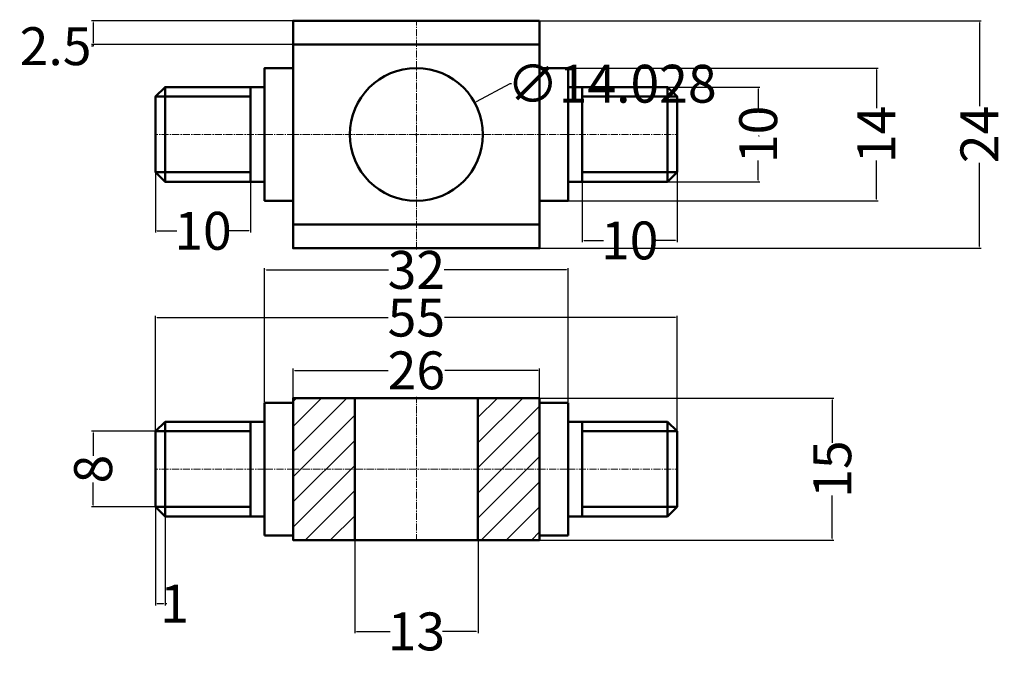
# Model space of a CAD drawing. Units: millimetres. Extents: x 37 to 141, y 13 to 80.
import ezdxf

# ---------------------------------------------------------------- set-up
doc = ezdxf.new("R2010")
doc.units = ezdxf.units.MM
doc.header["$MEASUREMENT"] = 0
doc.linetypes.add('CENTER2', pattern=[1.125, 0.75, -0.125, 0.125, -0.125])
for name, color, linetype, lineweight in [('M-CNTR', 4, 'CENTER2', 18), ('M-DIMS', 2, 'Continuous', 25), ('M-HATC', 8, 'Continuous', 18), ('M-OUTL', 7, 'Continuous', 50), ('M-TEXT', 7, 'Continuous', 25)]:
    doc.layers.add(name, color=color, linetype=linetype, lineweight=lineweight)
doc.styles.get("Standard").update_dxf_attribs({"font": 'arial.ttf'})
doc.dimstyles.get("Standard").update_dxf_attribs({"dimtxt": 4, "dimasz": 0.18, "dimexe": 0.18, "dimexo": 0.0625, "dimgap": 0.09, "dimtad": 0, "dimtoh": 1, "dimdec": 0, "dimzin": 0, "dimdsep": 46, "dimtxsty": 'Standard', "dimcen": 0.09, "dimadec": 0, "dimazin": 0, "dimtfac": 1, "dimtdec": 0, "dimtofl": 0, "dimtmove": 0, "dimatfit": 3, "dimfxl": 1, "dimtolj": 1, "dimtzin": 0, "dimarcsym": 0})

# ---------------------------------------------------------------- blocks, each defined once
blk = doc.blocks.new('*U1')
at = {"layer": 'M-CNTR', "color": 0, "transparency": 16777216}
blk.add_line((-1.62, 0), (1.62, 0), dxfattribs=at)
blk = doc.blocks.new('*U2')
at = {"layer": 'M-CNTR', "color": 0, "transparency": 16777216}
blk.add_line((0, -12.12), (0, 12.12), dxfattribs=at)
blk = doc.blocks.new('*U3')
at = {"layer": 'M-CNTR', "color": 0, "transparency": 16777216}
blk.add_line((-13.12, 0), (13.12, 0), dxfattribs=at)
blk = doc.blocks.new('*U4')
at = {"layer": 'M-CNTR', "color": 0, "transparency": 16777216}
blk.add_line((1.62, 0), (-1.62, 0), dxfattribs=at)
blk = doc.blocks.new('*U5')
at = {"layer": 'M-CNTR', "color": 0, "transparency": 16777216}
blk.add_line((1.62, 0), (-1.62, 0), dxfattribs=at)
blk = doc.blocks.new('*U6')
at = {"layer": 'M-CNTR', "color": 0, "transparency": 16777216}
blk.add_line((-1.62, 0), (1.62, 0), dxfattribs=at)
blk = doc.blocks.new('*U7')
at = {"layer": 'M-CNTR', "color": 0, "transparency": 16777216}
blk.add_line((-13.12, 0), (13.12, 0), dxfattribs=at)
blk = doc.blocks.new('*D8')
at = {"layer": 'Defpoints', "color": 0, "transparency": 16777216}
for p in [(78.94, 39.78), (78.94, 24.78), (122.8, 24.78)]:
    blk.add_point(p, dxfattribs=at)
at = {"layer": 'M-DIMS', "color": 0, "lineweight": -2, "transparency": 16777216}
for p, q in [((79, 39.78), (122.98, 39.78)), ((122.8, 39.6), (122.8, 35.06)), ((122.8, 24.96), (122.8, 29.5)), ((79, 24.78), (122.98, 24.78))]:
    blk.add_line(p, q, dxfattribs=at)
at = {"layer": 'M-DIMS', "color": 0, "transparency": 16777216}
for points in [[(122.77, 39.6), (122.83, 39.6), (122.8, 39.78)], [(122.77, 24.96), (122.83, 24.96), (122.8, 24.78)]]:
    blk.add_solid(points, dxfattribs=at)
at = {"layer": 'M-DIMS', "color": 0, "transparency": 16777216, "insert": (122.8, 32.28), "char_height": 4, "attachment_point": 5, "rotation": 90}
blk.add_mtext('\\A1;15', dxfattribs=at)
blk = doc.blocks.new('*D9')
at = {"layer": 'Defpoints', "color": 0, "transparency": 16777216}
for p in [(106.44, 48.27), (51.44, 32.28), (106.44, 32.28)]:
    blk.add_point(p, dxfattribs=at)
at = {"layer": 'M-DIMS', "color": 0, "lineweight": -2, "transparency": 16777216}
for p, q in [((51.44, 32.34), (51.44, 48.45)), ((51.62, 48.27), (75.97, 48.27)), ((106.26, 48.27), (81.91, 48.27)), ((106.44, 32.34), (106.44, 48.45))]:
    blk.add_line(p, q, dxfattribs=at)
at = {"layer": 'M-DIMS', "color": 0, "transparency": 16777216}
for points in [[(51.62, 48.3), (51.62, 48.24), (51.44, 48.27)], [(106.26, 48.3), (106.26, 48.24), (106.44, 48.27)]]:
    blk.add_solid(points, dxfattribs=at)
at = {"layer": 'M-DIMS', "color": 0, "transparency": 16777216, "insert": (78.94, 48.27), "char_height": 4, "attachment_point": 5}
blk.add_mtext('\\A1;55', dxfattribs=at)
blk = doc.blocks.new('*D10')
at = {"layer": 'Defpoints', "color": 0, "transparency": 16777216}
for p in [(94.94, 53.3), (62.94, 39.28), (94.94, 39.28)]:
    blk.add_point(p, dxfattribs=at)
at = {"layer": 'M-DIMS', "color": 0, "lineweight": -2, "transparency": 16777216}
for p, q in [((62.94, 39.34), (62.94, 53.48)), ((63.12, 53.3), (76.01, 53.3)), ((94.76, 53.3), (81.87, 53.3)), ((94.94, 39.34), (94.94, 53.48))]:
    blk.add_line(p, q, dxfattribs=at)
at = {"layer": 'M-DIMS', "color": 0, "transparency": 16777216}
for points in [[(63.12, 53.33), (63.12, 53.27), (62.94, 53.3)], [(94.76, 53.33), (94.76, 53.27), (94.94, 53.3)]]:
    blk.add_solid(points, dxfattribs=at)
at = {"layer": 'M-DIMS', "color": 0, "transparency": 16777216, "insert": (78.94, 53.3), "char_height": 4, "attachment_point": 5}
blk.add_mtext('\\A1;32', dxfattribs=at)
blk = doc.blocks.new('*D11')
at = {"layer": 'Defpoints', "color": 0, "transparency": 16777216}
for p in [(91.94, 42.7), (65.94, 39.78), (91.94, 39.78)]:
    blk.add_point(p, dxfattribs=at)
at = {"layer": 'M-DIMS', "color": 0, "lineweight": -2, "transparency": 16777216}
for p, q in [((65.94, 39.84), (65.94, 42.88)), ((66.12, 42.7), (75.95, 42.7)), ((91.76, 42.7), (81.93, 42.7)), ((91.94, 39.84), (91.94, 42.88))]:
    blk.add_line(p, q, dxfattribs=at)
at = {"layer": 'M-DIMS', "color": 0, "transparency": 16777216}
for points in [[(66.12, 42.73), (66.12, 42.67), (65.94, 42.7)], [(91.76, 42.73), (91.76, 42.67), (91.94, 42.7)]]:
    blk.add_solid(points, dxfattribs=at)
at = {"layer": 'M-DIMS', "color": 0, "transparency": 16777216, "insert": (78.94, 42.7), "char_height": 4, "attachment_point": 5}
blk.add_mtext('\\A1;26', dxfattribs=at)
blk = doc.blocks.new('*D12')
at = {"layer": 'Defpoints', "color": 0, "transparency": 16777216}
for p in [(72.44, 24.78), (85.44, 24.78), (85.44, 15.15)]:
    blk.add_point(p, dxfattribs=at)
at = {"layer": 'M-DIMS', "color": 0, "lineweight": -2, "transparency": 16777216}
for p, q in [((72.44, 24.72), (72.44, 14.97)), ((85.44, 24.72), (85.44, 14.97)), ((72.62, 15.15), (76.17, 15.15)), ((85.26, 15.15), (81.7, 15.15))]:
    blk.add_line(p, q, dxfattribs=at)
at = {"layer": 'M-DIMS', "color": 0, "transparency": 16777216}
for points in [[(72.62, 15.18), (72.62, 15.12), (72.44, 15.15)], [(85.26, 15.18), (85.26, 15.12), (85.44, 15.15)]]:
    blk.add_solid(points, dxfattribs=at)
at = {"layer": 'M-DIMS', "color": 0, "transparency": 16777216, "insert": (78.94, 15.15), "char_height": 4, "attachment_point": 5}
blk.add_mtext('\\A1;13', dxfattribs=at)
blk = doc.blocks.new('*D13')
at = {"layer": 'Defpoints', "color": 0, "transparency": 16777216}
for p in [(51.44, 63.6), (61.44, 63.6), (61.44, 57.43)]:
    blk.add_point(p, dxfattribs=at)
at = {"layer": 'M-DIMS', "color": 0, "lineweight": -2, "transparency": 16777216}
for p, q in [((51.44, 63.54), (51.44, 57.25)), ((61.44, 63.54), (61.44, 57.25)), ((51.62, 57.43), (53.68, 57.43)), ((61.26, 57.43), (59.2, 57.43))]:
    blk.add_line(p, q, dxfattribs=at)
at = {"layer": 'M-DIMS', "color": 0, "transparency": 16777216}
for points in [[(51.62, 57.46), (51.62, 57.4), (51.44, 57.43)], [(61.26, 57.46), (61.26, 57.4), (61.44, 57.43)]]:
    blk.add_solid(points, dxfattribs=at)
at = {"layer": 'M-DIMS', "color": 0, "transparency": 16777216, "insert": (56.44, 57.43), "char_height": 4, "attachment_point": 5}
blk.add_mtext('\\A1;10', dxfattribs=at)
blk = doc.blocks.new('*D14')
at = {"layer": 'Defpoints', "color": 0, "transparency": 16777216}
for p in [(96.44, 63.6), (106.44, 63.6), (106.44, 56.41)]:
    blk.add_point(p, dxfattribs=at)
at = {"layer": 'M-DIMS', "color": 0, "lineweight": -2, "transparency": 16777216}
for p, q in [((96.44, 63.54), (96.44, 56.23)), ((106.44, 63.54), (106.44, 56.23)), ((96.62, 56.41), (98.68, 56.41)), ((106.26, 56.41), (104.2, 56.41))]:
    blk.add_line(p, q, dxfattribs=at)
at = {"layer": 'M-DIMS', "color": 0, "transparency": 16777216}
for points in [[(96.62, 56.44), (96.62, 56.38), (96.44, 56.41)], [(106.26, 56.44), (106.26, 56.38), (106.44, 56.41)]]:
    blk.add_solid(points, dxfattribs=at)
at = {"layer": 'M-DIMS', "color": 0, "transparency": 16777216, "insert": (101.44, 56.41), "char_height": 4, "attachment_point": 5}
blk.add_mtext('\\A1;10', dxfattribs=at)
blk = doc.blocks.new('*D15')
at = {"layer": 'Defpoints', "color": 0, "transparency": 16777216}
for p in [(94.94, 74.6), (94.94, 60.6), (127.45, 60.6)]:
    blk.add_point(p, dxfattribs=at)
at = {"layer": 'M-DIMS', "color": 0, "lineweight": -2, "transparency": 16777216}
for p, q in [((95, 74.6), (127.63, 74.6)), ((127.45, 74.42), (127.45, 70.36)), ((127.45, 60.78), (127.45, 64.84)), ((95, 60.6), (127.63, 60.6))]:
    blk.add_line(p, q, dxfattribs=at)
at = {"layer": 'M-DIMS', "color": 0, "transparency": 16777216}
for points in [[(127.42, 74.42), (127.48, 74.42), (127.45, 74.6)], [(127.42, 60.78), (127.48, 60.78), (127.45, 60.6)]]:
    blk.add_solid(points, dxfattribs=at)
at = {"layer": 'M-DIMS', "color": 0, "transparency": 16777216, "insert": (127.45, 67.6), "char_height": 4, "attachment_point": 5, "rotation": 90}
blk.add_mtext('\\A1;14', dxfattribs=at)
blk = doc.blocks.new('*D16')
at = {"layer": 'Defpoints', "color": 0, "transparency": 16777216}
for p in [(91.94, 79.59), (91.94, 55.59), (138.32, 55.59)]:
    blk.add_point(p, dxfattribs=at)
at = {"layer": 'M-DIMS', "color": 0, "lineweight": -2, "transparency": 16777216}
for p, q in [((92, 79.59), (138.5, 79.59)), ((138.32, 79.41), (138.32, 70.57)), ((138.32, 55.77), (138.32, 64.61)), ((92, 55.59), (138.5, 55.59))]:
    blk.add_line(p, q, dxfattribs=at)
at = {"layer": 'M-DIMS', "color": 0, "transparency": 16777216}
for points in [[(138.29, 79.41), (138.35, 79.41), (138.32, 79.59)], [(138.29, 55.77), (138.35, 55.77), (138.32, 55.59)]]:
    blk.add_solid(points, dxfattribs=at)
at = {"layer": 'M-DIMS', "color": 0, "transparency": 16777216, "insert": (138.32, 67.59), "char_height": 4, "attachment_point": 5, "rotation": 90}
blk.add_mtext('\\A1;24', dxfattribs=at)
blk = doc.blocks.new('*D17')
at = {"layer": 'Defpoints', "color": 0, "transparency": 16777216}
for p in [(105.44, 72.6), (105.44, 62.6), (114.99, 62.6)]:
    blk.add_point(p, dxfattribs=at)
at = {"layer": 'M-DIMS', "color": 0, "lineweight": -2, "transparency": 16777216}
for p, q in [((105.5, 72.6), (115.17, 72.6)), ((114.99, 72.42), (114.99, 70.36)), ((114.99, 62.78), (114.99, 64.84)), ((105.5, 62.6), (115.17, 62.6))]:
    blk.add_line(p, q, dxfattribs=at)
at = {"layer": 'M-DIMS', "color": 0, "transparency": 16777216}
for points in [[(114.96, 72.42), (115.02, 72.42), (114.99, 72.6)], [(114.96, 62.78), (115.02, 62.78), (114.99, 62.6)]]:
    blk.add_solid(points, dxfattribs=at)
at = {"layer": 'M-DIMS', "color": 0, "transparency": 16777216, "insert": (114.99, 67.6), "char_height": 4, "attachment_point": 5, "rotation": 90}
blk.add_mtext('\\A1;10', dxfattribs=at)
blk = doc.blocks.new('TRUNNION-END-M10')
for p, q in [((0, 7), (-3, 7)), ((-3, 7), (-3, -7)), ((-13.5, 5), (-14.5, 4)), ((-3, 5), (-13.5, 5)), ((-13.5, 5), (-13.5, -5)), ((-4.5, 5), (-4.5, -5)), ((-14.5, 4), (-14.5, -4)), ((-14.5, 4), (-4.5, 4)), ((-13.5, -5), (-14.5, -4)), ((-14.5, -4), (-4.5, -4)), ((-3, -5), (-13.5, -5)), ((-3, -7), (0, -7))]:
    blk.add_line(p, q)
blk = doc.blocks.new('*D19')
at = {"layer": 'Defpoints', "color": 0, "transparency": 16777216}
for p in [(65.94, 79.59), (44.85, 77.09), (65.94, 77.09)]:
    blk.add_point(p, dxfattribs=at)
at = {"layer": 'M-DIMS', "color": 0, "lineweight": -2, "transparency": 16777216}
for p, q in [((65.88, 79.59), (44.67, 79.59)), ((44.85, 79.41), (44.85, 77.27)), ((65.88, 77.09), (44.67, 77.09)), ((44.85, 76.91), (44.67, 76.91)), ((44.85, 77.09), (44.85, 76.91))]:
    blk.add_line(p, q, dxfattribs=at)
at = {"layer": 'M-DIMS', "color": 0, "transparency": 16777216}
for points in [[(44.82, 79.41), (44.88, 79.41), (44.85, 79.59)], [(44.82, 77.27), (44.88, 77.27), (44.85, 77.09)]]:
    blk.add_solid(points, dxfattribs=at)
at = {"layer": 'M-DIMS', "color": 0, "transparency": 16777216, "insert": (40.89, 76.91), "char_height": 4, "attachment_point": 5}
blk.add_mtext('\\A1;2.5', dxfattribs=at)
blk = doc.blocks.new('*D20')
at = {"layer": 'Defpoints', "color": 0, "transparency": 16777216}
for p in [(51.44, 28.28), (52.44, 27.28), (52.44, 18.08)]:
    blk.add_point(p, dxfattribs=at)
at = {"layer": 'M-DIMS', "color": 0, "lineweight": -2, "transparency": 16777216}
for p, q in [((51.44, 28.22), (51.44, 17.9)), ((52.44, 27.22), (52.44, 17.9)), ((51.62, 18.08), (52.26, 18.08)), ((52.44, 18.08), (52.62, 18.08))]:
    blk.add_line(p, q, dxfattribs=at)
at = {"layer": 'M-DIMS', "color": 0, "transparency": 16777216}
for points in [[(51.62, 18.11), (51.62, 18.05), (51.44, 18.08)], [(52.26, 18.11), (52.26, 18.05), (52.44, 18.08)]]:
    blk.add_solid(points, dxfattribs=at)
at = {"layer": 'M-DIMS', "color": 0, "transparency": 16777216, "insert": (53.44, 18.08), "char_height": 4, "attachment_point": 5}
blk.add_mtext('\\A1;1', dxfattribs=at)
blk = doc.blocks.new('*D21')
at = {"layer": 'Defpoints', "color": 0, "transparency": 16777216}
for p in [(44.85, 36.28), (51.44, 36.28), (51.44, 28.28)]:
    blk.add_point(p, dxfattribs=at)
at = {"layer": 'M-DIMS', "color": 0, "lineweight": -2, "transparency": 16777216}
for p, q in [((51.38, 36.28), (44.67, 36.28)), ((44.85, 36.1), (44.85, 33.69)), ((44.85, 28.46), (44.85, 30.87)), ((51.38, 28.28), (44.67, 28.28))]:
    blk.add_line(p, q, dxfattribs=at)
at = {"layer": 'M-DIMS', "color": 0, "transparency": 16777216}
for points in [[(44.82, 36.1), (44.88, 36.1), (44.85, 36.28)], [(44.82, 28.46), (44.88, 28.46), (44.85, 28.28)]]:
    blk.add_solid(points, dxfattribs=at)
at = {"layer": 'M-DIMS', "color": 0, "transparency": 16777216, "insert": (44.85, 32.28), "char_height": 4, "attachment_point": 5, "rotation": 90}
blk.add_mtext('\\A1;8', dxfattribs=at)
blk = doc.blocks.new('*D22')
at = {"layer": 'Defpoints', "color": 0, "transparency": 16777216}
for p in [(85.1, 70.94), (72.78, 64.24)]:
    blk.add_point(p, dxfattribs=at)
at = {"layer": 'M-DIMS', "color": 0, "lineweight": -2, "transparency": 16777216}
for p, q in [((88.8, 72.95), (85.26, 71.03)), ((88.98, 72.95), (88.8, 72.95)), ((78.85, 67.59), (79.03, 67.59)), ((78.94, 67.5), (78.94, 67.68))]:
    blk.add_line(p, q, dxfattribs=at)
at = {"layer": 'M-DIMS', "color": 0, "transparency": 16777216}
blk.add_solid([(85.24, 71.05), (85.27, 71), (85.1, 70.94)], dxfattribs=at)
at = {"layer": 'M-DIMS', "color": 0, "transparency": 16777216, "insert": (99.55, 72.95), "char_height": 4, "attachment_point": 5}
blk.add_mtext('\\A1;∅14.028', dxfattribs=at)

msp = doc.modelspace()

# ---------------------------------------------------------------- hatches: boundary and pattern name
at = {"layer": 'M-HATC'}
h = msp.add_hatch(dxfattribs=at)
h.set_pattern_fill('ANSI31', color=256, scale=15)
h.paths.add_polyline_path([(72.4381, 39.7818), (65.9381, 39.7818), (65.9381, 24.7818), (72.4381, 24.7818)])
h.paths.add_polyline_path([(91.9381, 39.7818), (85.4381, 39.7818), (85.4381, 24.7818), (91.9381, 24.7818)])

# ---------------------------------------------------------------- linework, layer by layer
at = {"layer": 'M-CNTR'}
for p, q in [((78.9381, 79.5893), (78.9381, 79.7093)), ((62.9381, 67.6033), (51.4381, 67.6033)), ((65.8181, 67.5893), (65.9381, 67.5893)), ((91.9381, 67.5893), (92.0581, 67.5893)), ((94.9381, 67.6033), (106.4381, 67.6033)), ((78.9381, 55.4693), (78.9381, 55.5893)), ((78.9381, 24.6618), (78.9381, 39.9018)), ((62.9381, 32.2818), (51.4381, 32.2818)), ((94.9381, 32.2818), (106.4381, 32.2818))]:
    msp.add_line(p, q, dxfattribs=at)
at = {"layer": 'M-OUTL'}
for p, q in [((94.9381, 72.6033), (105.4381, 72.6033)), ((96.4381, 72.6033), (96.4381, 62.6033)), ((51.4381, 71.6033), (51.4381, 63.6033)), ((106.4381, 71.6033), (106.4381, 63.6033)), ((62.9381, 62.6033), (61.4381, 62.6033)), ((72.4381, 24.7818), (72.4381, 39.7818)), ((85.4381, 39.7818), (85.4381, 24.7818))]:
    msp.add_line(p, q, dxfattribs=at)
for points in [[(91.9381, 79.5893), (91.9381, 55.5893), (65.9381, 55.5893), (65.9381, 79.5893)], [(91.9381, 39.7818), (91.9381, 24.7818), (65.9381, 24.7818), (65.9381, 39.7818)]]:
    msp.add_lwpolyline(points, close=True, dxfattribs=at)
for points in [[(65.9381, 77.0893), (91.9381, 77.0893)], [(65.9381, 74.6033), (62.9381, 74.6033), (62.9381, 60.6033), (65.9381, 60.6033)], [(91.9381, 74.6033), (94.9381, 74.6033), (94.9381, 60.6033), (91.9381, 60.6033)], [(62.9381, 72.6033), (61.4381, 72.6033), (52.4381, 72.6033), (52.4381, 62.6033), (51.4381, 63.6033), (61.4381, 63.6033)], [(52.4381, 72.6033), (51.4381, 71.6033), (61.4381, 71.6033)], [(52.4381, 62.6033), (61.4381, 62.6033), (61.4381, 72.6033)], [(96.4381, 71.6033), (106.4381, 71.6033), (105.4381, 72.6033), (105.4381, 62.6033), (94.9381, 62.6033)], [(105.4381, 62.6033), (106.4381, 63.6033), (96.4381, 63.6033)], [(91.9381, 58.0893), (65.9381, 58.0893)]]:
    msp.add_lwpolyline(points, dxfattribs=at)
msp.add_circle((78.9381, 67.5893), 7.014, dxfattribs=at)

# ---------------------------------------------------------------- block references
at = {"layer": 'M-CNTR'}
for name, p in [('*U2', (78.9381, 67.5893)), ('*U4', (64.4381, 67.6033)), ('*U3', (78.9381, 67.5893)), ('*U1', (93.4381, 67.6033)), ('*U5', (64.4381, 32.2818)), ('*U7', (78.9381, 32.2818)), ('*U6', (93.4381, 32.2818))]:
    msp.add_blockref(name, p, dxfattribs=at)
at = {"layer": 'M-OUTL'}
msp.add_blockref('TRUNNION-END-M10', (65.9381, 32.2818), dxfattribs=at)
at = {"layer": 'M-OUTL', "rotation": 180}
msp.add_blockref('TRUNNION-END-M10', (91.9381, 32.2818), dxfattribs=at)

# ---------------------------------------------------------------- texts
at = {"layer": 'M-TEXT'}
msp.add_attdef('M', (114.9938, 67.34), '', height=0.2, dxfattribs=at)

# ---------------------------------------------------------------- dimensions: what is measured, and where the dimension line sits
at = {"layer": 'M-DIMS'}
for base, p1, p2, override, picture, middle in [((44.8531, 77.0893), (65.9381, 79.5893), (65.9381, 77.0893), {"dimdec": 1, "dimlfac": 1, "dimrnd": 0, "dimzin": 0, "dimdsep": 46, "dimlunit": 2}, '*D19', (40.8928, 76.9093)), ((138.321, 55.5893), (91.9381, 79.5893), (91.9381, 55.5893), {"dimclrd": 0, "dimclre": 0, "dimclrt": 0}, '*D16', (138.321, 67.5893)), ((127.4543, 60.6033), (94.9381, 74.6033), (94.9381, 60.6033), {"dimclrd": 0, "dimclre": 0, "dimclrt": 0}, '*D15', (127.4543, 67.6033)), ((114.9938, 62.6033), (105.4381, 72.6033), (105.4381, 62.6033), {"dimclrd": 0, "dimclre": 0, "dimclrt": 0}, '*D17', (114.9938, 67.6033)), ((122.8026, 24.7818), (78.9381, 39.7818), (78.9381, 24.7818), {"dimclrd": 0, "dimclre": 0, "dimclrt": 0}, '*D8', (122.8026, 32.2818)), ((44.8531, 36.2818), (51.4381, 28.2818), (51.4381, 36.2818), {"dimdec": 0, "dimlfac": 1, "dimrnd": 0, "dimzin": 0, "dimdsep": 46, "dimlunit": 2}, '*D21', (44.8531, 32.2818))]:
    dim = msp.add_linear_dim(base=base, p1=p1, p2=p2, angle=90, dimstyle='Standard', override=override, dxfattribs=at)
    dim.commit()
    dim.dimension.update_dxf_attribs({"geometry": picture, "text_midpoint": middle})
dim = msp.add_diameter_dim_2p(p1=(72.7762, 64.2385), p2=(85.1, 70.94), dimstyle='Standard', override={"dimdec": 3, "dimlfac": 1, "dimrnd": 0, "dimzin": 0, "dimdsep": 46, "dimlunit": 2}, dxfattribs=at)
dim.commit()
dim.dimension.update_dxf_attribs({"geometry": '*D22', "text_midpoint": (99.5501, 72.9505), "dimtype": 163})
for base, p1, p2, override, picture, middle in [((61.4381, 57.4275), (51.4381, 63.6033), (61.4381, 63.6033), {"dimclrd": 0, "dimclre": 0, "dimclrt": 0}, '*D13', (56.4381, 57.4275)), ((106.4381, 56.4055), (96.4381, 63.6033), (106.4381, 63.6033), {"dimclrd": 0, "dimclre": 0, "dimclrt": 0}, '*D14', (101.4381, 56.4055)), ((94.9381, 53.2988), (62.9381, 39.2818), (94.9381, 39.2818), {"dimclrd": 0, "dimclre": 0, "dimclrt": 0}, '*D10', (78.9381, 53.2988)), ((106.4381, 48.2665), (51.4381, 32.2818), (106.4381, 32.2818), {"dimclrd": 0, "dimclre": 0, "dimclrt": 0}, '*D9', (78.9381, 48.2665)), ((91.9381, 42.7045), (65.9381, 39.7818), (91.9381, 39.7818), {"dimclrd": 0, "dimclre": 0, "dimclrt": 0}, '*D11', (78.9381, 42.7045)), ((52.4381, 18.0768), (51.4381, 28.2818), (52.4381, 27.2818), {"dimdec": 0, "dimlfac": 1, "dimrnd": 0, "dimzin": 0, "dimdsep": 46, "dimlunit": 2}, '*D20', (53.4448, 18.0768)), ((85.4381, 15.146), (72.4381, 24.7818), (85.4381, 24.7818), {"dimclrd": 0, "dimclre": 0, "dimclrt": 0}, '*D12', (78.9381, 15.146))]:
    dim = msp.add_linear_dim(base=base, p1=p1, p2=p2, dimstyle='Standard', override=override, dxfattribs=at)
    dim.commit()
    dim.dimension.update_dxf_attribs({"geometry": picture, "text_midpoint": middle})

doc.saveas('drawing.dxf')
